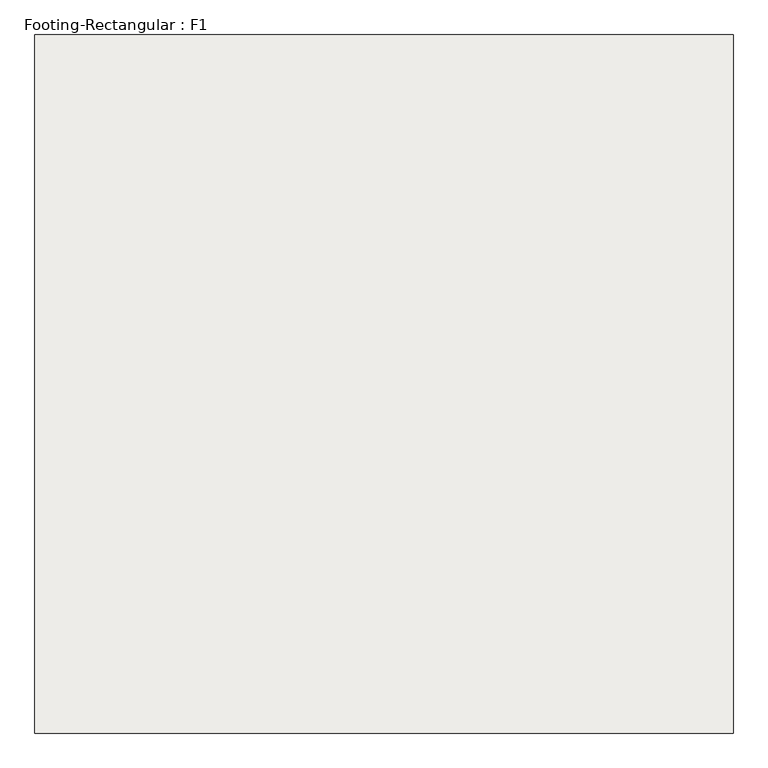
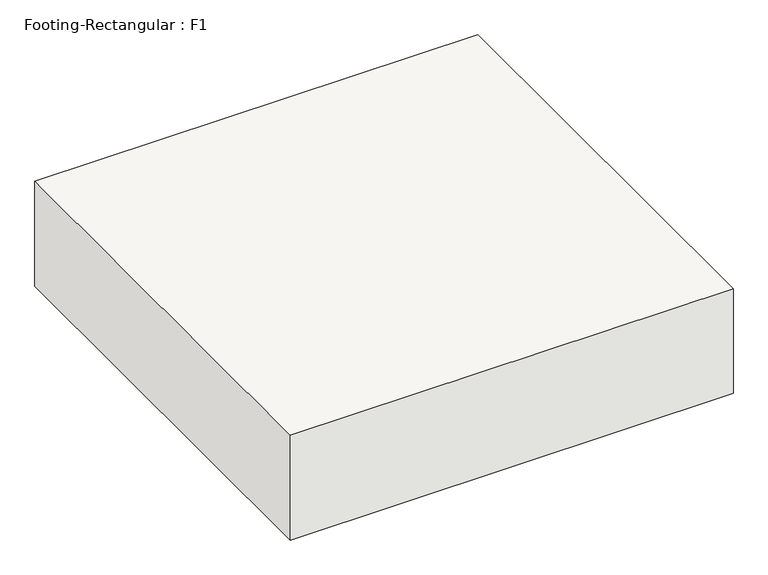
"""IFC4 building model written with IfcOpenShell, lengths in millimetres: slab geometry, Footing-Rectangular : F1."""

from ifc_helpers import new_model, si_unit, frame, origin, place, context, project, spatial, polyline, outline, extrude, source, transform, mapped, element, save


def footing_rectangular_f1_8f1f0fab(model_context):
    return source(origin(), model_context, "Body", "SweptSolid", [
        extrude(outline(polyline([(1066.8, 1066.8), (1066.8, -1066.8), (-1066.8, -1066.8), (-1066.8, 1066.8), (1066.8, 1066.8)])), frame((0.0, 0.0, -533.4), z_axis=(0.0, 0.0, 1.0), x_axis=(1.0, 0.0, 0.0)), (0.0, 0.0, 1.0), 533.4),
    ])


if __name__ == "__main__":
    model = new_model("IFC4")
    model_context = context("Model", 3, world=origin())
    ifc_project = project(units=[si_unit("LENGTHUNIT", "METRE", prefix="MILLI")], contexts=[model_context])
    site = spatial("IfcSite", under=ifc_project)
    building = spatial("IfcBuilding", under=site)
    placement = place(None, origin())
    footing_rectangular_f1_shape = footing_rectangular_f1_8f1f0fab(model_context)
    element("IfcSlab", 1, ObjectType="Footing-Rectangular : F1", at=placement, inside=building, context=model_context, shape_type="MappedRepresentation", body=[
        mapped(footing_rectangular_f1_shape, transform((0.0, 0.0, 0.0), x_axis=(1.0, 0.0, 0.0), y_axis=(0.0, 1.0, 0.0), z_axis=(0.0, 0.0, 1.0))),
    ])
    save(model, "model.ifc")

# Revit data of these elements
# Type "Footing-Rectangular : F1"
#   Width = 2133.6 mm
#   Length = 2133.6 mm
#   Foundation Thickness = 533.4 mm
#   Structural Material [instance default] = Concrete - Cast-in-Place Concrete
#   Assembly Code = ""
# Element 1 (IfcSlab, "Footing-Rectangular : F1")
#   Materials on its faces: "Concrete - Cast-in-Place Concrete"
# Materials
#   "Concrete - Cast-in-Place Concrete": class "Concrete", colour RGB 192 192 192, transparency 0, Cost = 0
